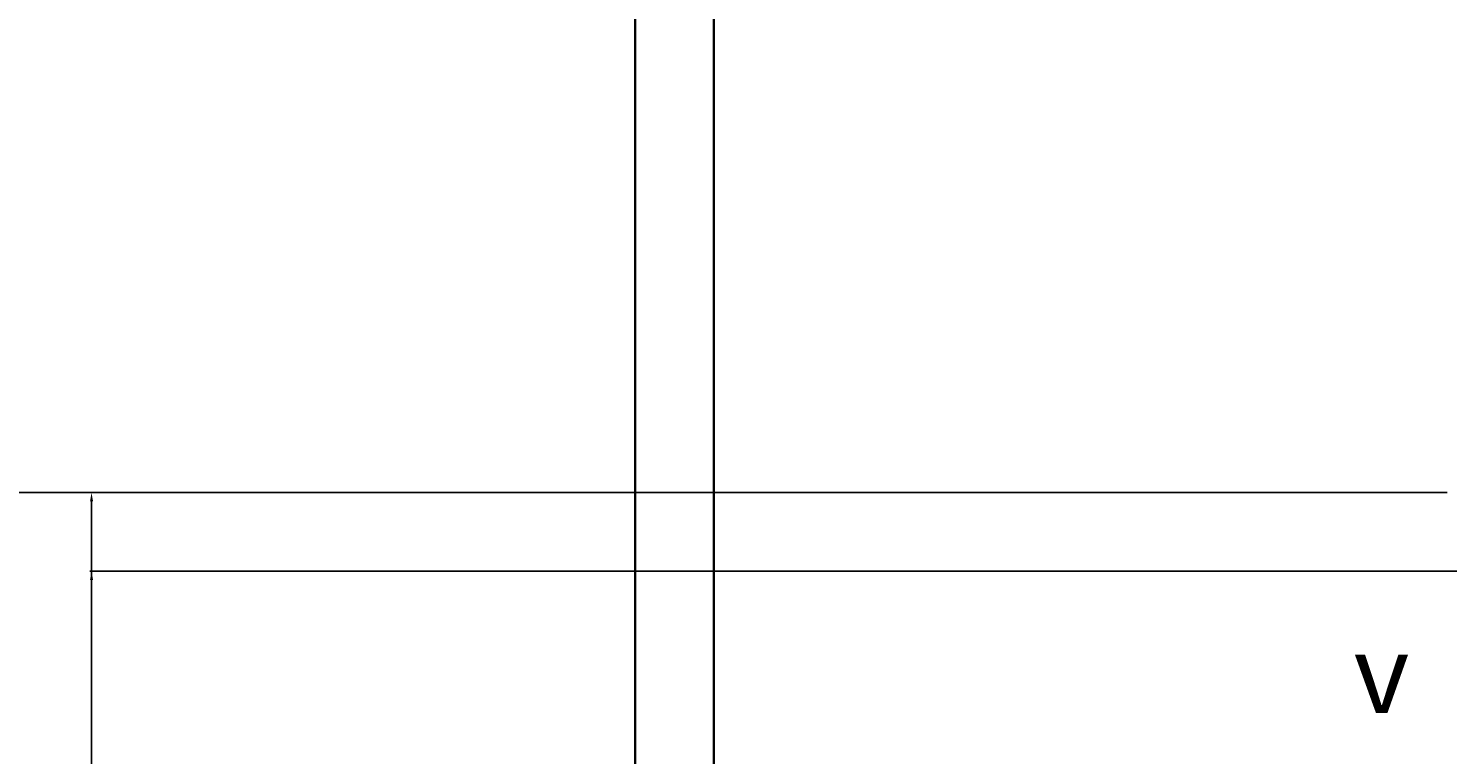
# Model space of a CAD drawing. Units: inches. Extents: x -364 to 705, y -52 to 1250.
# Tile 24 of 34: x -134 to 29, y 956 to 1039. Entities that reach past the tile are written whole.
import ezdxf

# ---------------------------------------------------------------- set-up
doc = ezdxf.new("R2010")
doc.units = ezdxf.units.IN
doc.header["$MEASUREMENT"] = 0
for name, color, linetype, lineweight in [('A-ANNO-DIMS', 4, 'Continuous', 18), ('A-ANNO-IDEN', 1, 'Continuous', 18), ('C-WALL', 41, 'Continuous', 35)]:
    doc.layers.add(name, color=color, linetype=linetype, lineweight=lineweight)
doc.styles.get("Standard").update_dxf_attribs({"font": 'arial.ttf'})
doc.dimstyles.get("Standard").update_dxf_attribs({"dimtxt": 1, "dimasz": 1, "dimexe": 0.18, "dimexo": 0.0625, "dimgap": 0.09, "dimtad": 0, "dimtih": 1, "dimtoh": 1, "dimdec": 0, "dimzin": 0, "dimdsep": 46, "dimlunit": 3, "dimtxsty": 'Standard', "dimcen": 0.09, "dimadec": 0, "dimazin": 0, "dimtfac": 1, "dimtdec": 0, "dimtofl": 0, "dimtmove": 0, "dimatfit": 3, "dimfxl": 1, "dimtolj": 1, "dimtzin": 0, "dimarcsym": 0})

# ---------------------------------------------------------------- blocks, each defined once
blk = doc.blocks.new('*D19')
at = {"layer": 'A-ANNO-DIMS', "color": 0, "lineweight": -2, "transparency": 16777216}
for p, q in [((28.52, 986.11), (-248.33, 986.11)), ((-248.15, 985.11), (-248.15, 574.22)), ((-248.15, 149.87), (-248.15, 560.77)), ((28.52, 148.87), (-248.33, 148.87))]:
    blk.add_line(p, q, dxfattribs=at)
at = {"layer": 'A-ANNO-DIMS', "color": 0, "transparency": 16777216}
for points in [[(-248.32, 985.11), (-247.99, 985.11), (-248.15, 986.11)], [(-248.32, 149.87), (-247.99, 149.87), (-248.15, 148.87)]]:
    blk.add_solid(points, dxfattribs=at)
at = {"layer": 'Defpoints', "color": 0, "transparency": 16777216}
for p in [(28.58, 986.11), (-248.15, 148.87), (28.58, 148.87)]:
    blk.add_point(p, dxfattribs=at)
at = {"layer": 'A-ANNO-DIMS', "color": 0, "transparency": 16777216, "insert": (-248.15, 567.49), "char_height": 1, "attachment_point": 5}
blk.add_mtext('\\A1;{\\H13x;69\'-9"}', dxfattribs=at)
blk = doc.blocks.new('*D20')
at = {"layer": 'A-ANNO-DIMS', "color": 0, "lineweight": -2, "transparency": 16777216}
for p, q in [((28.52, 986.11), (-188.21, 986.11)), ((-188.03, 985.11), (-188.03, 917.23)), ((-188.03, 836.11), (-188.03, 904)), ((37.52, 835.11), (-188.21, 835.11))]:
    blk.add_line(p, q, dxfattribs=at)
at = {"layer": 'A-ANNO-DIMS', "color": 0, "transparency": 16777216}
for points in [[(-188.19, 985.11), (-187.86, 985.11), (-188.03, 986.11)], [(-188.19, 836.11), (-187.86, 836.11), (-188.03, 835.11)]]:
    blk.add_solid(points, dxfattribs=at)
at = {"layer": 'Defpoints', "color": 0, "transparency": 16777216}
for p in [(28.58, 986.11), (-188.03, 835.11), (37.58, 835.11)]:
    blk.add_point(p, dxfattribs=at)
at = {"layer": 'A-ANNO-DIMS', "color": 0, "transparency": 16777216, "insert": (-188.03, 910.61), "char_height": 1, "attachment_point": 5}
blk.add_mtext('\\A1;{\\H13x;12\'-7"}', dxfattribs=at)
blk = doc.blocks.new('*D76')
at = {"layer": 'A-ANNO-DIMS', "color": 0, "lineweight": -2, "transparency": 16777216}
for p, q in [((28.52, 986.11), (-126.85, 986.11)), ((-126.67, 985.11), (-126.67, 499.22)), ((-126.67, 12.11), (-126.67, 498.01)), ((28.52, 11.11), (-126.85, 11.11))]:
    blk.add_line(p, q, dxfattribs=at)
at = {"layer": 'A-ANNO-DIMS', "color": 0, "transparency": 16777216}
for points in [[(-126.84, 985.11), (-126.5, 985.11), (-126.67, 986.11)], [(-126.84, 12.11), (-126.5, 12.11), (-126.67, 11.11)]]:
    blk.add_solid(points, dxfattribs=at)
at = {"layer": 'Defpoints', "color": 0, "transparency": 16777216}
for p in [(-126.67, 986.11), (28.58, 986.11), (28.58, 11.11)]:
    blk.add_point(p, dxfattribs=at)
at = {"layer": 'A-ANNO-DIMS', "color": 0, "transparency": 16777216, "insert": (-126.67, 498.61), "char_height": 1, "attachment_point": 5}
blk.add_mtext('\\A1;81\'-3"', dxfattribs=at)
blk = doc.blocks.new('*D93')
at = {"layer": 'A-ANNO-DIMS', "color": 0, "lineweight": -2, "transparency": 16777216}
for p, q in [((37.52, 977.11), (-126.85, 977.11)), ((-126.67, 976.11), (-126.67, 954.22)), ((-126.67, 931.11), (-126.67, 953.01)), ((37.52, 930.11), (-126.85, 930.11))]:
    blk.add_line(p, q, dxfattribs=at)
at = {"layer": 'A-ANNO-DIMS', "color": 0, "transparency": 16777216}
for points in [[(-126.84, 976.11), (-126.5, 976.11), (-126.67, 977.11)], [(-126.84, 931.11), (-126.5, 931.11), (-126.67, 930.11)]]:
    blk.add_solid(points, dxfattribs=at)
at = {"layer": 'Defpoints', "color": 0, "transparency": 16777216}
for p in [(37.58, 977.11), (-126.67, 930.11), (37.58, 930.11)]:
    blk.add_point(p, dxfattribs=at)
at = {"layer": 'A-ANNO-DIMS', "color": 0, "transparency": 16777216, "insert": (-126.67, 953.61), "char_height": 1, "attachment_point": 5}
blk.add_mtext('\\A1;3\'-11"', dxfattribs=at)

msp = doc.modelspace()

# ---------------------------------------------------------------- linework, layer by layer
at = {"layer": 'C-WALL'}
for p, q in [((-64.42, 11.11), (-64.42, 1079.11)), ((-55.42, 11.11), (-55.42, 1070.11))]:
    msp.add_line(p, q, dxfattribs=at)

# ---------------------------------------------------------------- texts
at = {"layer": 'A-ANNO-IDEN', "insert": (17.81, 969.88), "char_height": 9, "attachment_point": 1}
msp.add_mtext_dynamic_manual_height_columns('v', width=10.6887, gutter_width=1, heights=[0], dxfattribs=at)

# ---------------------------------------------------------------- dimensions: what is measured, and where the dimension line sits
at = {"layer": 'A-ANNO-DIMS'}
dim = msp.add_linear_dim(base=(-248.15, 148.87), p1=(28.58, 986.11), p2=(28.58, 148.87), angle=90, text='{\\H13x;<>}', dimstyle='Standard', override={"dimclrd": 0, "dimclre": 0, "dimclrt": 0}, dxfattribs=at)
dim.commit()
dim.dimension.update_dxf_attribs({"geometry": '*D19', "text_midpoint": (-248.15, 567.49)})
dim = msp.add_linear_dim(base=(-188.03, 835.11), p1=(28.58, 986.11), p2=(37.58, 835.11), angle=90, text='{\\H13x;<>}', dimstyle='Standard', override={"dimclrd": 0, "dimclre": 0, "dimclrt": 0}, dxfattribs=at)
dim.commit()
dim.dimension.update_dxf_attribs({"geometry": '*D20', "text_midpoint": (-188.03, 910.61), "dimtype": 160})
for base, p1, p2, picture, middle in [((-126.67, 986.11), (28.58, 11.11), (28.58, 986.11), '*D76', (-126.67, 498.61)), ((-126.67, 930.11), (37.58, 977.11), (37.58, 930.11), '*D93', (-126.67, 953.61))]:
    dim = msp.add_linear_dim(base=base, p1=p1, p2=p2, angle=90, dimstyle='Standard', override={"dimdec": 1, "dimlfac": 1, "dimrnd": 0, "dimzin": 1, "dimdsep": 46, "dimlunit": 4, "dimfrac": 2}, dxfattribs=at)
    dim.commit()
    dim.dimension.update_dxf_attribs({"geometry": picture, "text_midpoint": middle})

doc.saveas('drawing.dxf')
